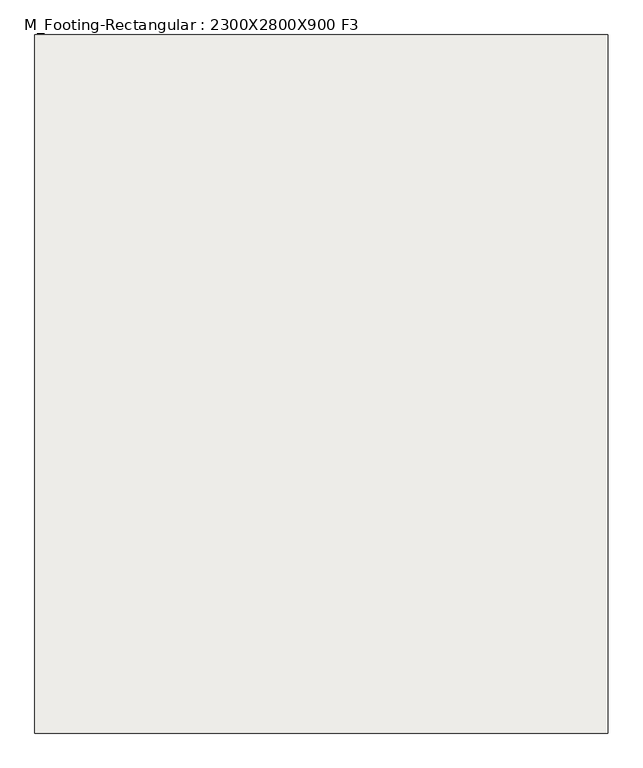
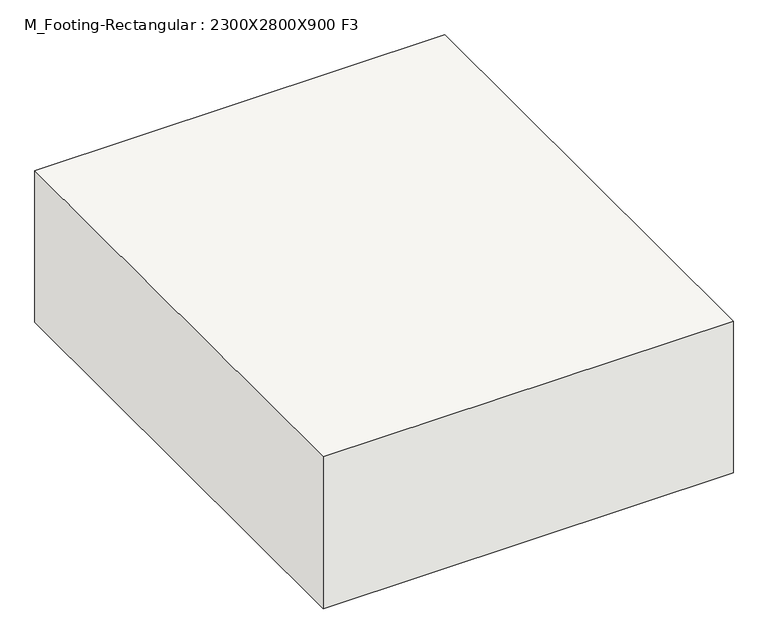
"""IFC4 building model written with IfcOpenShell, lengths in millimetres: slab geometry, M_Footing-Rectangular : 2300X2800X900 F3."""

from ifc_helpers import new_model, si_unit, frame, origin, place, context, project, spatial, polyline, outline, extrude, source, transform, mapped, element, save


def m_footing_rectangular_2300x2800x900_f3_c46bdd4c(model_context):
    return source(origin(), model_context, "Body", "SweptSolid", [
        extrude(outline(polyline([(1150.0, 1400.0), (1150.0, -1400.0), (-1150.0, -1400.0), (-1150.0, 1400.0), (1150.0, 1400.0)])), frame((0.0, 0.0, -900.0), z_axis=(0.0, 0.0, 1.0), x_axis=(1.0, 0.0, 0.0)), (0.0, 0.0, 1.0), 900.0),
    ])


if __name__ == "__main__":
    model = new_model("IFC4")
    model_context = context("Model", 3, world=origin())
    ifc_project = project(units=[si_unit("LENGTHUNIT", "METRE", prefix="MILLI")], contexts=[model_context])
    site = spatial("IfcSite", under=ifc_project)
    building = spatial("IfcBuilding", under=site)
    placement = place(None, origin())
    m_footing_rectangular_2300x2800x900_f3_shape = m_footing_rectangular_2300x2800x900_f3_c46bdd4c(model_context)
    element("IfcSlab", 1, ObjectType="M_Footing-Rectangular : 2300X2800X900 F3", at=placement, inside=building, context=model_context, shape_type="MappedRepresentation", body=[
        mapped(m_footing_rectangular_2300x2800x900_f3_shape, transform((0.0, 0.0, 0.0), x_axis=(1.0, 0.0, 0.0), y_axis=(0.0, 1.0, 0.0), z_axis=(0.0, 0.0, 1.0))),
    ])
    save(model, "model.ifc")

# Revit data of these elements
# Type "M_Footing-Rectangular : 2300X2800X900 F3"
#   Width = 2300 mm
#   Length = 2800 mm
#   Foundation Thickness = 900 mm
#   Structural Material [instance default] = Concrete, Cast-in-Place gray
#   Assembly Code = ""
# Element 1 (IfcSlab, "M_Footing-Rectangular : 2300X2800X900 F3")
#   Structural Material = Concrete, Cast In Situ
#   Materials on its faces: "Concrete, Cast In Situ"
# Materials
#   "Concrete, Cast-in-Place gray": class "Concrete", colour RGB 192 192 192, transparency 0, Description = "Cast-in-place concrete", Cost = 0
#   "Concrete, Cast In Situ": class "Concrete", colour RGB 192 192 192, transparency 0, Description = "physical material", Cost = 0
